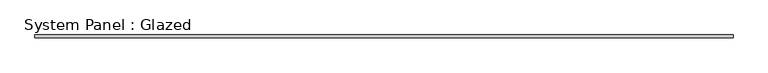
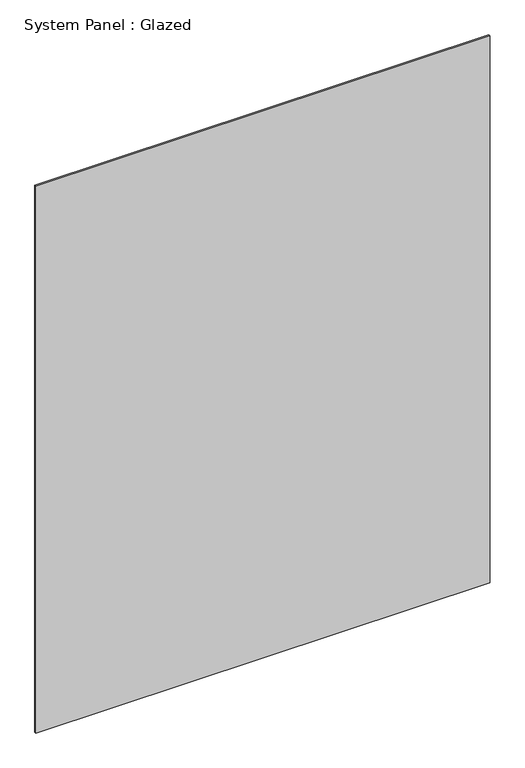
"""IFC4 building model written with IfcOpenShell, lengths in millimetres: plate geometry, System Panel : Glazed."""

from ifc_helpers import new_model, si_unit, origin, origin_with_axes, place, context, project, spatial, polyline, outline, extrude, source, transform, mapped, element, save


def system_panel_glazed_393e2e5d(model_context):
    return source(origin(), model_context, "Body", "SweptSolid", [
        extrude(outline(polyline([(733.3333332, 34.0), (-733.3333332, 34.0), (-733.3333332, 40.0), (733.3333332, 40.0), (733.3333332, 34.0)])), origin_with_axes(), (0.0, 0.0, 1.0), 1865.4113705),
    ])


if __name__ == "__main__":
    model = new_model("IFC4")
    model_context = context("Model", 3, world=origin())
    ifc_project = project(units=[si_unit("LENGTHUNIT", "METRE", prefix="MILLI")], contexts=[model_context])
    site = spatial("IfcSite", under=ifc_project)
    building = spatial("IfcBuilding", under=site)
    placement = place(None, origin())
    system_panel_glazed_shape = system_panel_glazed_393e2e5d(model_context)
    element("IfcPlate", 1, ObjectType="System Panel : Glazed", at=placement, inside=building, context=model_context, shape_type="MappedRepresentation", body=[
        mapped(system_panel_glazed_shape, transform((0.0, 0.0, 0.0), x_axis=(1.0, 0.0, 0.0), y_axis=(0.0, 1.0, 0.0), z_axis=(0.0, 0.0, 1.0))),
    ])
    save(model, "model.ifc")

# Revit data of these elements
# Type "System Panel : Glazed"
#   Construction Type Id = "GSP4R"
#   Analytic Construction = "1/8 in Pilkington single glazing"
#   Visual Light Transmittance = 0.9
#   Solar Heat Gain Coefficient = 0.86
#   Heat Transfer Coefficient (U) = 6.7069 W/(m²·K)
#   Define Thermal Properties by = 1
# Element 1 (IfcPlate, "System Panel : Glazed")
#   Materials on its faces: "Default New Material(6)"
# Materials
#   "Default New Material(6)": class "Generic", colour RGB 191 25 25, transparency 0.9, Cost = 0
